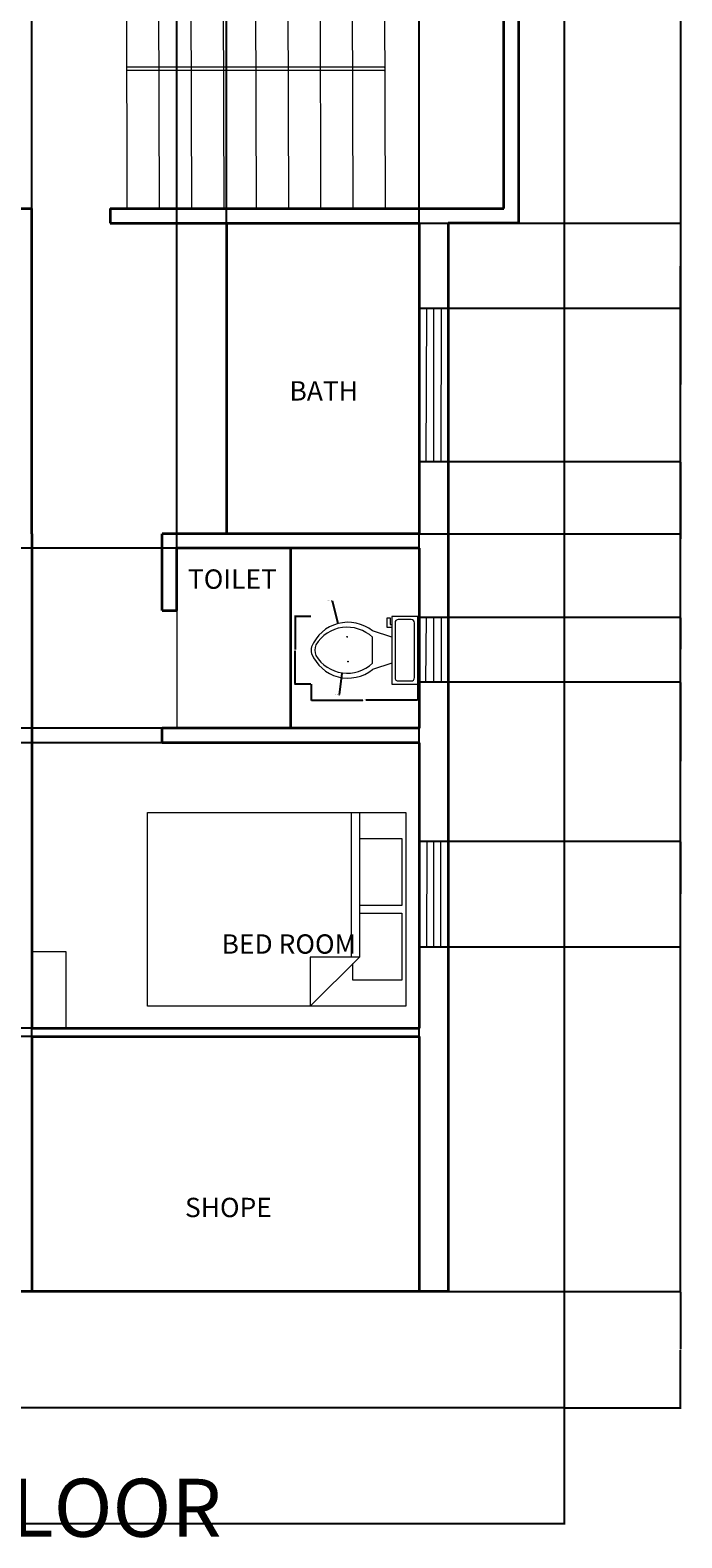
# Model space of a CAD drawing. Units: inches. Extents: x 2621 to 3621, y 1701 to 2465.
# Tile 2 of 6: x 2888 to 3090, y 1701 to 2169. Entities that reach past the tile are written whole.
import ezdxf

# ---------------------------------------------------------------- set-up
doc = ezdxf.new("R2010")
doc.units = ezdxf.units.IN
for name, color, linetype, lineweight in [('A-ANNO-DIMS', 2, 'Continuous', 18), ('A-ANNO-TEXT', 7, 'Continuous', 25), ('A-AREA-IDEN', 7, 'Continuous', 18), ('A-DOOR', 3, 'Continuous', 18), ('A-FLOR-CASE', 32, 'Continuous', 18), ('A-FLOR-FIXT', 9, 'Continuous', 18), ('A-FLOR-STRS', 30, 'Continuous', 18), ('A-FURN', 8, 'Continuous', 18), ('A-GLAZ', 4, 'Continuous', 18), ('A-WALL', 7, 'Continuous', 35), ('C-PROP', 8, 'Continuous', 25)]:
    doc.layers.add(name, color=color, linetype=linetype, lineweight=lineweight)
doc.styles.get("Standard").update_dxf_attribs({"font": 'arial.ttf'})
doc.dimstyles.get("Standard").update_dxf_attribs({"dimtxt": 0.18, "dimasz": 0.18, "dimexe": 0.18, "dimexo": 0.0625, "dimgap": 0.09, "dimtad": 0, "dimtih": 1, "dimtoh": 1, "dimdec": 4, "dimzin": 0, "dimdsep": 46, "dimtxsty": 'Standard', "dimcen": 0.09, "dimadec": 0, "dimazin": 0, "dimtfac": 1, "dimtdec": 4, "dimtofl": 0, "dimtmove": 0, "dimatfit": 3, "dimfxl": 1, "dimtolj": 1, "dimtzin": 0, "dimarcsym": 0})

# ---------------------------------------------------------------- blocks, each defined once
blk = doc.blocks.new('Bed - Queen')
for p, q in [((0, -80.00003), (0, 0)), ((0, 0), (59.99999, 0)), ((59.99999, 0), (59.99999, -80.00003)), ((7.99999, -1.2), (28.79998, -1.2)), ((7.99999, -14.4), (7.99999, -1.2)), ((28.79998, -1.2), (28.79998, -14.4)), ((31.19999, -1.2), (51.99999, -1.2)), ((31.19999, -14.4), (31.19999, -1.2)), ((51.99999, -1.2), (51.99999, -16.4)), ((0, -14.4), (44.8, -14.4)), ((44.8, -16.8), (0, -16.8)), ((59.99999, -29.6), (44.8, -14.4)), ((44.8, -14.4), (44.8, -29.6)), ((51.99999, -16.4), (46.79936, -16.4)), ((44.8, -29.6), (59.99999, -29.6)), ((59.99999, -80.00003), (0, -80.00003))]:
    blk.add_line(p, q)
blk = doc.blocks.new('Toilet - top')
for p, q in [((9.5, -6), (9.5, -2)), ((-10, -8.5), (-8, -8.5)), ((-10, -9.5), (-10, -8.5)), ((-8, -8.5), (-8, -8)), ((-7, -8), (-7, -9.5)), ((-4, -8), (-6, -14)), ((4, -8), (6, -14)), ((-7, -9.5), (-10, -9.5)), ((4, -14), (-4, -14))]:
    blk.add_line(p, q)
blk.add_lwpolyline([(10.5, -8), (10.5, 0), (-10.5, 0), (-10.5, -8)], close=True)
for points in [[(-9.5, -2), (-9.5, -6)], [(8.5, -1), (-8.5, -1)], [(-8.5, -7), (8.5, -7)]]:
    blk.add_lwpolyline(points)
for centre, radius, start, end in [((-8.62, -1.88), 0.884, 81.8699, 188.1301), ((8.62, -1.88), 0.884, 351.8699, 98.1301), ((-8.62, -6.12), 0.884, 171.8699, 278.1301), ((8.62, -6.12), 0.884, 261.8699, 8.1301), ((3.52, -21.58), 12.17, 141.4691, 247.9714), ((4.2, -21.82), 11.33, 136.3677, 238.9468), ((-3.52, -21.58), 12.17, 292.0284, 38.5307), ((-4.2, -21.82), 11.33, 301.053, 43.6321), ((0, -27.88), 4, 245.7318, 294.2682), ((0, -29), 4, 254.8605, 285.1395)]:
    blk.add_arc(centre, radius, start, end)
blk = doc.blocks.new('LOT-33X57')
for p, q in [((396, 684), (396, 0)), ((396, 0), (0, 0))]:
    blk.add_line(p, q)
blk = doc.blocks.new('STAIR-RETURN-FLIGHT')
for p, q in [((0.25, 0), (0, 86.58)), ((10.25, 0.03), (10, 86.61)), ((20.25, 0.06), (20, 86.64)), ((30.25, 0.09), (30, 86.67)), ((40.25, 0.12), (40, 86.7)), ((50.25, 0.15), (50, 86.73)), ((60.25, 0.18), (60, 86.76)), ((70.25, 0.2), (70, 86.79)), ((80.25, 0.23), (80, 86.82)), ((6.51, 44.03), (0.13, 44.03)), ((6.51, 43.03), (0.13, 43.03)), ((79.82, 44.03), (6.51, 44.03)), ((79.82, 43.03), (6.51, 43.03)), ((79.82, 44.03), (80.13, 44.03)), ((79.82, 43.03), (80.13, 43.03)), ((70.59, 0.23), (70.59, 0.06))]:
    blk.add_line(p, q)
blk = doc.blocks.new('*D33')
at = {"layer": 'A-ANNO-DIMS', "color": 0, "lineweight": -2, "transparency": 16777216}
for p, q in [((2975.04, 1965.73), (2975.04, 1960.65)), ((3008.09, 1965.73), (3008.09, 1960.65)), ((2975.22, 1960.83), (2991.1, 1960.83)), ((3007.91, 1960.83), (2992.03, 1960.83))]:
    blk.add_line(p, q, dxfattribs=at)
at = {"layer": 'A-ANNO-DIMS', "color": 0, "transparency": 16777216}
for points in [[(2975.22, 1960.86), (2975.22, 1960.8), (2975.04, 1960.83)], [(3007.91, 1960.86), (3007.91, 1960.8), (3008.09, 1960.83)]]:
    blk.add_solid(points, dxfattribs=at)
at = {"layer": 'Defpoints', "color": 0, "transparency": 16777216}
for p in [(2975.04, 1965.79), (3008.09, 1965.79), (3008.09, 1960.83)]:
    blk.add_point(p, dxfattribs=at)
at = {"layer": 'A-ANNO-DIMS', "color": 0, "transparency": 16777216, "insert": (2991.57, 1960.83), "char_height": 0.18, "attachment_point": 5}
blk.add_mtext('\\A1;WC 33', dxfattribs=at)
blk = doc.blocks.new('*D34')
at = {"layer": 'A-ANNO-DIMS', "color": 0, "lineweight": -2, "transparency": 16777216}
for p, q in [((2974.98, 1986.79), (2969.91, 1986.79)), ((2970.09, 1986.61), (2970.09, 1976.47)), ((2970.09, 1965.97), (2970.09, 1976.11)), ((2974.98, 1965.79), (2969.91, 1965.79))]:
    blk.add_line(p, q, dxfattribs=at)
at = {"layer": 'A-ANNO-DIMS', "color": 0, "transparency": 16777216}
for points in [[(2970.06, 1986.61), (2970.12, 1986.61), (2970.09, 1986.79)], [(2970.06, 1965.97), (2970.12, 1965.97), (2970.09, 1965.79)]]:
    blk.add_solid(points, dxfattribs=at)
at = {"layer": 'Defpoints', "color": 0, "transparency": 16777216}
for p in [(2975.04, 1986.79), (2970.09, 1965.79), (2975.04, 1965.79)]:
    blk.add_point(p, dxfattribs=at)
at = {"layer": 'A-ANNO-DIMS', "color": 0, "transparency": 16777216, "insert": (2970.09, 1976.29), "char_height": 0.18, "attachment_point": 5}
blk.add_mtext('\\A1;21', dxfattribs=at)
blk = doc.blocks.new('*D35')
at = {"layer": 'A-ANNO-DIMS', "color": 0, "lineweight": -2, "transparency": 16777216}
for p, q in [((2657.52, 1741.34), (2657.52, 1705.2)), ((3053.52, 1741.34), (3053.52, 1705.2)), ((2657.7, 1705.38), (2855.23, 1705.38)), ((3053.34, 1705.38), (2855.81, 1705.38))]:
    blk.add_line(p, q, dxfattribs=at)
at = {"layer": 'A-ANNO-DIMS', "color": 0, "transparency": 16777216}
for points in [[(2657.7, 1705.41), (2657.7, 1705.35), (2657.52, 1705.38)], [(3053.34, 1705.41), (3053.34, 1705.35), (3053.52, 1705.38)]]:
    blk.add_solid(points, dxfattribs=at)
at = {"layer": 'Defpoints', "color": 0, "transparency": 16777216}
for p in [(2657.52, 1741.4), (3053.52, 1741.4), (3053.52, 1705.38)]:
    blk.add_point(p, dxfattribs=at)
at = {"layer": 'A-ANNO-DIMS', "color": 0, "transparency": 16777216, "insert": (2855.52, 1705.38), "char_height": 0.18, "attachment_point": 5}
blk.add_mtext('\\A1;396', dxfattribs=at)
blk = doc.blocks.new('*D38')
at = {"layer": 'A-ANNO-DIMS', "color": 0, "lineweight": -2, "transparency": 16777216}
for p, q in [((3017.58, 2389.4), (3089.72, 2389.4)), ((3089.54, 2389.22), (3089.54, 2083.58)), ((3089.54, 1777.58), (3089.54, 2083.22)), ((3017.58, 1777.4), (3089.72, 1777.4))]:
    blk.add_line(p, q, dxfattribs=at)
at = {"layer": 'A-ANNO-DIMS', "color": 0, "transparency": 16777216}
for points in [[(3089.51, 2389.22), (3089.57, 2389.22), (3089.54, 2389.4)], [(3089.51, 1777.58), (3089.57, 1777.58), (3089.54, 1777.4)]]:
    blk.add_solid(points, dxfattribs=at)
at = {"layer": 'Defpoints', "color": 0, "transparency": 16777216}
for p in [(3017.52, 2389.4), (3089.54, 2389.4), (3017.52, 1777.4)]:
    blk.add_point(p, dxfattribs=at)
at = {"layer": 'A-ANNO-DIMS', "color": 0, "transparency": 16777216, "insert": (3089.54, 2083.4), "char_height": 0.18, "attachment_point": 5}
blk.add_mtext('\\A1;612', dxfattribs=at)
blk = doc.blocks.new('*D40')
at = {"layer": 'A-ANNO-DIMS', "color": 0, "lineweight": -2, "transparency": 16777216}
for p, q in [((3017.58, 1777.4), (3089.72, 1777.4)), ((3089.54, 1777.22), (3089.54, 1759.58)), ((3089.54, 1741.58), (3089.54, 1759.22)), ((3053.58, 1741.4), (3089.72, 1741.4))]:
    blk.add_line(p, q, dxfattribs=at)
at = {"layer": 'A-ANNO-DIMS', "color": 0, "transparency": 16777216}
for points in [[(3089.51, 1777.22), (3089.57, 1777.22), (3089.54, 1777.4)], [(3089.51, 1741.58), (3089.57, 1741.58), (3089.54, 1741.4)]]:
    blk.add_solid(points, dxfattribs=at)
at = {"layer": 'Defpoints', "color": 0, "transparency": 16777216}
for p in [(3017.52, 1777.4), (3089.54, 1777.4), (3053.52, 1741.4)]:
    blk.add_point(p, dxfattribs=at)
at = {"layer": 'A-ANNO-DIMS', "color": 0, "transparency": 16777216, "insert": (3089.54, 1759.4), "char_height": 0.18, "attachment_point": 5}
blk.add_mtext('\\A1;36', dxfattribs=at)
blk = doc.blocks.new('*D53')
at = {"layer": 'A-ANNO-DIMS', "color": 0, "lineweight": -2, "transparency": 16777216}
for p, q in [((2888.5, 1777.46), (2888.5, 2461.61)), ((2888.68, 2461.43), (2948.05, 2461.43)), ((3008.34, 2461.43), (2948.96, 2461.43)), ((3008.52, 1777.46), (3008.52, 2461.61))]:
    blk.add_line(p, q, dxfattribs=at)
at = {"layer": 'A-ANNO-DIMS', "color": 0, "transparency": 16777216}
for points in [[(2888.68, 2461.46), (2888.68, 2461.4), (2888.5, 2461.43)], [(3008.34, 2461.46), (3008.34, 2461.4), (3008.52, 2461.43)]]:
    blk.add_solid(points, dxfattribs=at)
at = {"layer": 'Defpoints', "color": 0, "transparency": 16777216}
for p in [(3008.52, 2461.43), (2888.5, 1777.4), (3008.52, 1777.4)]:
    blk.add_point(p, dxfattribs=at)
at = {"layer": 'A-ANNO-DIMS', "color": 0, "transparency": 16777216, "insert": (2948.51, 2461.43), "char_height": 0.18, "attachment_point": 5}
blk.add_mtext('\\A1;120.02', dxfattribs=at)
blk = doc.blocks.new('*D54')
at = {"layer": 'A-ANNO-DIMS', "color": 0, "lineweight": -2, "transparency": 16777216}
for p, q in [((3008.46, 1856.54), (2621.31, 1856.54)), ((2621.49, 1856.36), (2621.49, 1817.15)), ((2621.49, 1777.58), (2621.49, 1816.79)), ((3008.46, 1777.4), (2621.31, 1777.4))]:
    blk.add_line(p, q, dxfattribs=at)
at = {"layer": 'A-ANNO-DIMS', "color": 0, "transparency": 16777216}
for points in [[(2621.46, 1856.36), (2621.52, 1856.36), (2621.49, 1856.54)], [(2621.46, 1777.58), (2621.52, 1777.58), (2621.49, 1777.4)]]:
    blk.add_solid(points, dxfattribs=at)
at = {"layer": 'Defpoints', "color": 0, "transparency": 16777216}
for p in [(2621.49, 1856.54), (3008.52, 1856.54), (3008.52, 1777.4)]:
    blk.add_point(p, dxfattribs=at)
at = {"layer": 'A-ANNO-DIMS', "color": 0, "transparency": 16777216, "insert": (2621.49, 1816.97), "char_height": 0.18, "attachment_point": 5}
blk.add_mtext('\\A1;79.14', dxfattribs=at)
blk = doc.blocks.new('*D55')
at = {"layer": 'A-ANNO-DIMS', "color": 0, "lineweight": -2, "transparency": 16777216}
for p, q in [((3008.46, 1947.58), (2621.31, 1947.58)), ((2621.49, 1947.4), (2621.49, 1903.51)), ((2621.49, 1859.26), (2621.49, 1903.15)), ((3008.46, 1859.08), (2621.31, 1859.08))]:
    blk.add_line(p, q, dxfattribs=at)
at = {"layer": 'A-ANNO-DIMS', "color": 0, "transparency": 16777216}
for points in [[(2621.46, 1947.4), (2621.52, 1947.4), (2621.49, 1947.58)], [(2621.46, 1859.26), (2621.52, 1859.26), (2621.49, 1859.08)]]:
    blk.add_solid(points, dxfattribs=at)
at = {"layer": 'Defpoints', "color": 0, "transparency": 16777216}
for p in [(2621.49, 1947.58), (3008.52, 1947.58), (3008.52, 1859.08)]:
    blk.add_point(p, dxfattribs=at)
at = {"layer": 'A-ANNO-DIMS', "color": 0, "transparency": 16777216, "insert": (2621.49, 1903.33), "char_height": 0.18, "attachment_point": 5}
blk.add_mtext('\\A1;88.5', dxfattribs=at)
blk = doc.blocks.new('*D56')
at = {"layer": 'A-ANNO-DIMS', "color": 0, "lineweight": -2, "transparency": 16777216}
for p, q in [((2948.9, 2012.46), (2948.9, 2461.61)), ((2949.08, 2461.43), (2978.32, 2461.43)), ((3008.34, 2461.43), (2979.1, 2461.43)), ((3008.52, 2012.46), (3008.52, 2461.61))]:
    blk.add_line(p, q, dxfattribs=at)
at = {"layer": 'A-ANNO-DIMS', "color": 0, "transparency": 16777216}
for points in [[(2949.08, 2461.46), (2949.08, 2461.4), (2948.9, 2461.43)], [(3008.34, 2461.46), (3008.34, 2461.4), (3008.52, 2461.43)]]:
    blk.add_solid(points, dxfattribs=at)
at = {"layer": 'Defpoints', "color": 0, "transparency": 16777216}
for p in [(3008.52, 2461.43), (2948.9, 2012.4), (3008.52, 2012.4)]:
    blk.add_point(p, dxfattribs=at)
at = {"layer": 'A-ANNO-DIMS', "color": 0, "transparency": 16777216, "insert": (2978.71, 2461.43), "char_height": 0.18, "attachment_point": 5}
blk.add_mtext('\\A1;59.62', dxfattribs=at)
blk = doc.blocks.new('*D57')
at = {"layer": 'A-ANNO-DIMS', "color": 0, "lineweight": -2, "transparency": 16777216}
for p, q in [((2948.96, 2108.75), (3089.72, 2108.75)), ((3089.54, 2108.57), (3089.54, 2060.76)), ((3089.54, 2012.58), (3089.54, 2060.39)), ((2948.96, 2012.4), (3089.72, 2012.4))]:
    blk.add_line(p, q, dxfattribs=at)
at = {"layer": 'A-ANNO-DIMS', "color": 0, "transparency": 16777216}
for points in [[(3089.51, 2108.57), (3089.57, 2108.57), (3089.54, 2108.75)], [(3089.51, 2012.58), (3089.57, 2012.58), (3089.54, 2012.4)]]:
    blk.add_solid(points, dxfattribs=at)
at = {"layer": 'Defpoints', "color": 0, "transparency": 16777216}
for p in [(2948.9, 2108.75), (3089.54, 2108.75), (2948.9, 2012.4)]:
    blk.add_point(p, dxfattribs=at)
at = {"layer": 'A-ANNO-DIMS', "color": 0, "transparency": 16777216, "insert": (3089.54, 2060.58), "char_height": 0.18, "attachment_point": 5}
blk.add_mtext('\\A1;96.36', dxfattribs=at)
blk = doc.blocks.new('*D58')
at = {"layer": 'A-ANNO-DIMS', "color": 0, "lineweight": -2, "transparency": 16777216}
for p, q in [((2933.41, 2007.9), (2621.31, 2007.9)), ((2621.49, 2007.72), (2621.49, 1980.17)), ((2621.49, 1952.26), (2621.49, 1979.81)), ((2933.41, 1952.08), (2621.31, 1952.08))]:
    blk.add_line(p, q, dxfattribs=at)
at = {"layer": 'A-ANNO-DIMS', "color": 0, "transparency": 16777216}
for points in [[(2621.46, 2007.72), (2621.52, 2007.72), (2621.49, 2007.9)], [(2621.46, 1952.26), (2621.52, 1952.26), (2621.49, 1952.08)]]:
    blk.add_solid(points, dxfattribs=at)
at = {"layer": 'Defpoints', "color": 0, "transparency": 16777216}
for p in [(2621.49, 2007.9), (2933.47, 2007.9), (2933.47, 1952.08)]:
    blk.add_point(p, dxfattribs=at)
at = {"layer": 'A-ANNO-DIMS', "color": 0, "transparency": 16777216, "insert": (2621.49, 1979.99), "char_height": 0.18, "attachment_point": 5}
blk.add_mtext('\\A1;55.82', dxfattribs=at)
blk = doc.blocks.new('*D59')
at = {"layer": 'A-ANNO-DIMS', "color": 0, "lineweight": -2, "transparency": 16777216}
for p, q in [((2933.47, 2007.96), (2933.47, 2461.61)), ((2933.65, 2461.43), (2970.6, 2461.43)), ((3008.34, 2461.43), (2971.39, 2461.43)), ((3008.52, 2007.96), (3008.52, 2461.61))]:
    blk.add_line(p, q, dxfattribs=at)
at = {"layer": 'A-ANNO-DIMS', "color": 0, "transparency": 16777216}
for points in [[(2933.65, 2461.46), (2933.65, 2461.4), (2933.47, 2461.43)], [(3008.34, 2461.46), (3008.34, 2461.4), (3008.52, 2461.43)]]:
    blk.add_solid(points, dxfattribs=at)
at = {"layer": 'Defpoints', "color": 0, "transparency": 16777216}
for p in [(3008.52, 2461.43), (2933.47, 2007.9), (3008.52, 2007.9)]:
    blk.add_point(p, dxfattribs=at)
at = {"layer": 'A-ANNO-DIMS', "color": 0, "transparency": 16777216, "insert": (2971, 2461.43), "char_height": 0.18, "attachment_point": 5}
blk.add_mtext('\\A1;75.04', dxfattribs=at)
blk = doc.blocks.new('*D92')
at = {"layer": 'A-ANNO-DIMS', "color": 0, "lineweight": -2, "transparency": 16777216}
for p, q in [((3008.58, 1917.05), (3089.72, 1917.05)), ((3089.54, 1916.87), (3089.54, 1900.86)), ((3089.54, 1884.49), (3089.54, 1900.5)), ((3008.58, 1884.31), (3089.72, 1884.31))]:
    blk.add_line(p, q, dxfattribs=at)
at = {"layer": 'A-ANNO-DIMS', "color": 0, "transparency": 16777216}
for points in [[(3089.51, 1916.87), (3089.57, 1916.87), (3089.54, 1917.05)], [(3089.51, 1884.49), (3089.57, 1884.49), (3089.54, 1884.31)]]:
    blk.add_solid(points, dxfattribs=at)
at = {"layer": 'Defpoints', "color": 0, "transparency": 16777216}
for p in [(3008.52, 1917.05), (3089.54, 1917.05), (3008.52, 1884.31)]:
    blk.add_point(p, dxfattribs=at)
at = {"layer": 'A-ANNO-DIMS', "color": 0, "transparency": 16777216, "insert": (3089.54, 1900.68), "char_height": 0.18, "attachment_point": 5}
blk.add_mtext('\\A1;32.736', dxfattribs=at)
blk = doc.blocks.new('*D93')
at = {"layer": 'A-ANNO-DIMS', "color": 0, "lineweight": -2, "transparency": 16777216}
for p, q in [((3008.58, 1966.45), (3089.72, 1966.45)), ((3089.54, 1966.27), (3089.54, 1941.93)), ((3089.54, 1917.23), (3089.54, 1941.57)), ((3008.58, 1917.05), (3089.72, 1917.05))]:
    blk.add_line(p, q, dxfattribs=at)
at = {"layer": 'A-ANNO-DIMS', "color": 0, "transparency": 16777216}
for points in [[(3089.51, 1966.27), (3089.57, 1966.27), (3089.54, 1966.45)], [(3089.51, 1917.23), (3089.57, 1917.23), (3089.54, 1917.05)]]:
    blk.add_solid(points, dxfattribs=at)
at = {"layer": 'Defpoints', "color": 0, "transparency": 16777216}
for p in [(3008.52, 1966.45), (3089.54, 1966.45), (3008.52, 1917.05)]:
    blk.add_point(p, dxfattribs=at)
at = {"layer": 'A-ANNO-DIMS', "color": 0, "transparency": 16777216, "insert": (3089.54, 1941.75), "char_height": 0.18, "attachment_point": 5}
blk.add_mtext('\\A1;49.4', dxfattribs=at)
blk = doc.blocks.new('*D94')
at = {"layer": 'A-ANNO-DIMS', "color": 0, "lineweight": -2, "transparency": 16777216}
for p, q in [((3008.58, 1986.54), (3089.72, 1986.54)), ((3089.54, 1986.36), (3089.54, 1976.68)), ((3089.54, 1966.63), (3089.54, 1976.32)), ((3008.58, 1966.45), (3089.72, 1966.45))]:
    blk.add_line(p, q, dxfattribs=at)
at = {"layer": 'A-ANNO-DIMS', "color": 0, "transparency": 16777216}
for points in [[(3089.51, 1986.36), (3089.57, 1986.36), (3089.54, 1986.54)], [(3089.51, 1966.63), (3089.57, 1966.63), (3089.54, 1966.45)]]:
    blk.add_solid(points, dxfattribs=at)
at = {"layer": 'Defpoints', "color": 0, "transparency": 16777216}
for p in [(3008.52, 1986.54), (3089.54, 1986.54), (3008.52, 1966.45)]:
    blk.add_point(p, dxfattribs=at)
at = {"layer": 'A-ANNO-DIMS', "color": 0, "transparency": 16777216, "insert": (3089.54, 1976.5), "char_height": 0.18, "attachment_point": 5}
blk.add_mtext('\\A1;20.09', dxfattribs=at)
blk = doc.blocks.new('*D95')
at = {"layer": 'A-ANNO-DIMS', "color": 0, "lineweight": -2, "transparency": 16777216}
for p, q in [((3008.58, 2034.76), (3089.72, 2034.76)), ((3089.54, 2034.58), (3089.54, 2010.83)), ((3089.54, 1986.72), (3089.54, 2010.47)), ((3008.58, 1986.54), (3089.72, 1986.54))]:
    blk.add_line(p, q, dxfattribs=at)
at = {"layer": 'A-ANNO-DIMS', "color": 0, "transparency": 16777216}
for points in [[(3089.51, 2034.58), (3089.57, 2034.58), (3089.54, 2034.76)], [(3089.51, 1986.72), (3089.57, 1986.72), (3089.54, 1986.54)]]:
    blk.add_solid(points, dxfattribs=at)
at = {"layer": 'Defpoints', "color": 0, "transparency": 16777216}
for p in [(3008.52, 2034.76), (3089.54, 2034.76), (3008.52, 1986.54)]:
    blk.add_point(p, dxfattribs=at)
at = {"layer": 'A-ANNO-DIMS', "color": 0, "transparency": 16777216, "insert": (3089.54, 2010.65), "char_height": 0.18, "attachment_point": 5}
blk.add_mtext('\\A1;48.22', dxfattribs=at)
blk = doc.blocks.new('*D96')
at = {"layer": 'A-ANNO-DIMS', "color": 0, "lineweight": -2, "transparency": 16777216}
for p, q in [((3008.58, 2082.41), (3089.72, 2082.41)), ((3089.54, 2082.23), (3089.54, 2058.77)), ((3089.54, 2034.94), (3089.54, 2058.41)), ((3008.58, 2034.76), (3089.72, 2034.76))]:
    blk.add_line(p, q, dxfattribs=at)
at = {"layer": 'A-ANNO-DIMS', "color": 0, "transparency": 16777216}
for points in [[(3089.51, 2082.23), (3089.57, 2082.23), (3089.54, 2082.41)], [(3089.51, 2034.94), (3089.57, 2034.94), (3089.54, 2034.76)]]:
    blk.add_solid(points, dxfattribs=at)
at = {"layer": 'Defpoints', "color": 0, "transparency": 16777216}
for p in [(3008.52, 2082.41), (3089.54, 2082.41), (3008.52, 2034.76)]:
    blk.add_point(p, dxfattribs=at)
at = {"layer": 'A-ANNO-DIMS', "color": 0, "transparency": 16777216, "insert": (3089.54, 2058.59), "char_height": 0.18, "attachment_point": 5}
blk.add_mtext('\\A1;47.65', dxfattribs=at)
blk = doc.blocks.new('*D97')
at = {"layer": 'A-ANNO-DIMS', "color": 0, "lineweight": -2, "transparency": 16777216}
for p, q in [((3008.58, 2108.75), (3089.72, 2108.75)), ((3089.54, 2108.57), (3089.54, 2095.77)), ((3089.54, 2082.59), (3089.54, 2095.4)), ((3008.58, 2082.41), (3089.72, 2082.41))]:
    blk.add_line(p, q, dxfattribs=at)
at = {"layer": 'A-ANNO-DIMS', "color": 0, "transparency": 16777216}
for points in [[(3089.51, 2108.57), (3089.57, 2108.57), (3089.54, 2108.75)], [(3089.51, 2082.59), (3089.57, 2082.59), (3089.54, 2082.41)]]:
    blk.add_solid(points, dxfattribs=at)
at = {"layer": 'Defpoints', "color": 0, "transparency": 16777216}
for p in [(3008.52, 2108.75), (3089.54, 2108.75), (3008.52, 2082.41)]:
    blk.add_point(p, dxfattribs=at)
at = {"layer": 'A-ANNO-DIMS', "color": 0, "transparency": 16777216, "insert": (3089.54, 2095.58), "char_height": 0.18, "attachment_point": 5}
blk.add_mtext('\\A1;26.34', dxfattribs=at)
blk = doc.blocks.new('*D108')
at = {"layer": 'A-ANNO-DIMS', "color": 0, "lineweight": -2, "transparency": 16777216}
for p, q in [((2981.38, 1991.6), (2981.56, 1991.6)), ((2981.56, 1991.6), (2983.37, 1984.71)), ((2986.42, 1972.77), (2986.6, 1972.77)), ((2986.51, 1972.68), (2986.51, 1972.86))]:
    blk.add_line(p, q, dxfattribs=at)
at = {"layer": 'A-ANNO-DIMS', "color": 0, "transparency": 16777216}
blk.add_solid([(2983.4, 1984.72), (2983.34, 1984.71), (2983.42, 1984.54)], dxfattribs=at)
at = {"layer": 'Defpoints', "color": 0, "transparency": 16777216}
for p in [(2983.42, 1984.54), (2986.51, 1972.77)]:
    blk.add_point(p, dxfattribs=at)
at = {"layer": 'A-ANNO-DIMS', "color": 0, "transparency": 16777216, "insert": (2980.71, 1991.6), "char_height": 0.18, "attachment_point": 5}
blk.add_mtext('\\A1;2X R12.17', dxfattribs=at)
blk = doc.blocks.new('*D109')
at = {"layer": 'A-ANNO-DIMS', "color": 0, "lineweight": -2, "transparency": 16777216}
for p, q in [((2986.18, 1980.49), (2986.36, 1980.49)), ((2986.27, 1980.4), (2986.27, 1980.58)), ((2983.86, 1962.52), (2984.74, 1969.08)), ((2983.68, 1962.52), (2983.86, 1962.52))]:
    blk.add_line(p, q, dxfattribs=at)
at = {"layer": 'A-ANNO-DIMS', "color": 0, "transparency": 16777216}
blk.add_solid([(2984.71, 1969.09), (2984.77, 1969.08), (2984.76, 1969.26)], dxfattribs=at)
at = {"layer": 'Defpoints', "color": 0, "transparency": 16777216}
for p in [(2986.27, 1980.49), (2984.76, 1969.26)]:
    blk.add_point(p, dxfattribs=at)
at = {"layer": 'A-ANNO-DIMS', "color": 0, "transparency": 16777216, "insert": (2983, 1962.52), "char_height": 0.18, "attachment_point": 5}
blk.add_mtext('\\A1;2X R11.33', dxfattribs=at)

msp = doc.modelspace()

# ---------------------------------------------------------------- linework, layer by layer
at = {"layer": 'A-DOOR'}
msp.add_line((2933.4738, 1988.5937), (2933.4738, 1952.0771), dxfattribs=at)
at = {"layer": 'A-FLOR-CASE'}
msp.add_lwpolyline([(2888.495, 1859.0825), (2899.216, 1859.0825), (2899.216, 1882.7108), (2888.495, 1882.7108)], close=True, dxfattribs=at)
at = {"layer": 'A-GLAZ'}
for p, q in [((3010.7038, 2034.7604), (3010.9424, 2082.415)), ((3013.0184, 2082.415), (3013.0184, 2034.7604)), ((3015.3163, 2082.415), (3015.2368, 2034.7604)), ((3010.7349, 1986.5419), (3010.5077, 1966.4534)), ((3013.0184, 1986.5419), (3013.0184, 1966.4534)), ((3015.3938, 1986.5419), (3015.3938, 1966.4534)), ((3010.8891, 1917.049), (3010.7762, 1884.3132)), ((3013.0184, 1917.049), (3013.0184, 1884.3132)), ((3015.1972, 1917.049), (3015.1974, 1884.3132)), ((3008.5184, 1884.3132), (3017.5184, 1884.3132))]:
    msp.add_line(p, q, dxfattribs=at)
for points in [[(3008.5184, 2082.415), (3017.5184, 2082.415), (3017.5184, 2034.7604), (3008.5184, 2034.7604)], [(3008.5184, 1986.5419), (3017.5184, 1986.5419), (3017.5184, 1966.4534), (3008.5184, 1966.4534)], [(3008.5184, 1884.3132), (3017.5184, 1884.3132), (3017.5184, 1917.049), (3008.5184, 1917.049)]]:
    msp.add_lwpolyline(points, close=True, dxfattribs=at)
at = {"layer": 'A-WALL'}
for p, q in [((3039.3697, 2204.5707), (3039.3697, 2108.7527)), ((3034.7824, 2113.2527), (3034.7824, 2199.8382)), ((2883.995, 2113.2527), (2888.495, 2113.2527)), ((2888.495, 2012.3975), (2888.495, 2113.2527)), ((2912.8311, 2113.2527), (2912.8311, 2108.7527)), ((2912.8311, 2113.2527), (3017.5184, 2113.2527)), ((2912.8311, 2108.7527), (3008.5184, 2108.7527)), ((2948.9015, 2108.7527), (2948.9015, 2012.3975)), ((3008.5184, 2108.7527), (3008.5184, 2012.3975)), ((3017.5184, 2113.2527), (3034.7824, 2113.2527)), ((3039.3697, 2108.7527), (3017.5184, 2108.7527)), ((3017.5184, 2108.7527), (3017.5184, 1777.4015)), ((2888.495, 2012.3975), (2888.495, 2007.8975)), ((3008.5184, 2012.3975), (2928.9738, 2012.3975)), ((2928.9738, 2007.8975), (2928.9738, 2012.3975)), ((2888.495, 2007.8975), (2888.495, 1892.3987)), ((2928.9738, 1988.5937), (2928.9738, 2007.8975)), ((3008.5184, 2007.8975), (2933.4738, 2007.8975)), ((2933.4738, 1988.5937), (2933.4738, 2007.8975)), ((2968.7461, 1952.0771), (2968.7461, 2007.8975)), ((3008.5184, 2007.8975), (3008.5184, 1952.0771)), ((2928.9738, 1988.5937), (2933.4738, 1988.5937)), ((2928.9738, 1947.5771), (2928.9738, 1952.0771)), ((2933.4738, 1952.0771), (2928.9738, 1952.0771)), ((3008.5184, 1952.0771), (2933.4738, 1952.0771)), ((3008.5184, 1947.5771), (2928.9738, 1947.5771)), ((3008.5184, 1947.5771), (3008.5184, 1859.0825)), ((2888.495, 1892.3987), (2888.495, 1859.0825)), ((2888.495, 1859.0825), (3008.5184, 1859.0825)), ((2888.495, 1856.5401), (3008.5184, 1856.5401)), ((2888.495, 1856.5401), (2888.495, 1786.4015)), ((3008.5184, 1856.5401), (3008.5184, 1786.4015)), ((2888.495, 1786.4015), (2888.495, 1777.4015)), ((3008.5184, 1786.4015), (3008.5184, 1777.4015)), ((3017.5184, 1777.4015), (2883.995, 1777.4015))]:
    msp.add_line(p, q, dxfattribs=at)

# ---------------------------------------------------------------- block references
at = {"layer": 'A-FLOR-FIXT', "rotation": 270}
msp.add_blockref('Toilet - top', (3008.0882, 1976.2893), dxfattribs=at)
at = {"layer": 'A-FLOR-STRS'}
msp.add_blockref('STAIR-RETURN-FLIGHT', (2917.871, 2113.019), dxfattribs=at)
at = {"layer": 'A-FURN', "rotation": 270}
msp.add_blockref('Bed - Queen', (3004.4133, 1925.9517), dxfattribs=at)
at = {"layer": 'C-PROP'}
msp.add_blockref('LOT-33X57', (2657.518, 1741.402), dxfattribs=at)

# ---------------------------------------------------------------- texts
at = {"layer": 'A-ANNO-TEXT', "insert": (2759.8469, 1719.3538), "char_height": 18, "attachment_point": 1}
msp.add_mtext_dynamic_manual_height_columns('GROUND FLOOR', width=483.442651, gutter_width=12.5, heights=[0], dxfattribs=at)
at = {"layer": 'A-AREA-IDEN', "char_height": 6, "attachment_point": 1}
for s, width, insert in [('BATH', 12.444136, (2968.3648, 2059.7156)), ('TOILET', 9.68953, (2936.908, 2001.3427)), ('BED ROOM', 49.051461, (2947.3327, 1888.1756)), ('SHOPE', 21.347518, (2935.9947, 1806.4817))]:
    msp.add_mtext_dynamic_manual_height_columns(s, width=width, gutter_width=12.5, heights=[0], dxfattribs=dict(at, insert=insert))

# ---------------------------------------------------------------- dimensions: what is measured, and where the dimension line sits
at = {"layer": 'A-ANNO-DIMS'}
for base, p1, p2, override, picture, middle in [((3008.5184, 2461.427), (2888.495, 1777.4015), (3008.5184, 1777.4015), {"dimdec": 2, "dimlfac": 1, "dimrnd": 0, "dimzin": 0, "dimdsep": 46, "dimlunit": 2}, '*D53', (2948.5067, 2461.427)), ((3008.5184, 2461.427), (2933.4738, 2007.8975), (3008.5184, 2007.8975), {"dimdec": 2, "dimlfac": 1, "dimrnd": 0, "dimzin": 0, "dimdsep": 46, "dimlunit": 2}, '*D59', (2970.9961, 2461.427)), ((3008.5184, 2461.427), (2948.9015, 2012.3975), (3008.5184, 2012.3975), {"dimdec": 2, "dimlfac": 1, "dimrnd": 0, "dimzin": 0, "dimdsep": 46, "dimlunit": 2}, '*D56', (2978.71, 2461.427)), ((3053.5184, 1705.376), (2657.5184, 1741.4015), (3053.5184, 1741.4015), {"dimdec": 0, "dimlfac": 1, "dimrnd": 0, "dimzin": 0, "dimdsep": 46, "dimlunit": 2}, '*D35', (2855.5184, 1705.376))]:
    dim = msp.add_linear_dim(base=base, p1=p1, p2=p2, dimstyle='Standard', override=override, dxfattribs=at)
    dim.commit()
    dim.dimension.update_dxf_attribs({"geometry": picture, "text_midpoint": middle})
for base, p1, p2, angle, override, picture, middle in [((3089.5439, 2389.4015), (3017.5184, 1777.4015), (3017.5184, 2389.4015), 90, {"dimdec": 0, "dimlfac": 1, "dimrnd": 0, "dimzin": 0, "dimdsep": 46, "dimlunit": 2}, '*D38', (3089.5439, 2083.4015)), ((3089.5439, 2108.7527), (2948.9015, 2012.3975), (2948.9015, 2108.7527), 90, {"dimdec": 2, "dimlfac": 1, "dimrnd": 0, "dimzin": 0, "dimdsep": 46, "dimlunit": 2}, '*D57', (3089.5439, 2060.5751)), ((3089.5439, 2108.7527), (3008.5184, 2082.415), (3008.5184, 2108.7527), 90, {"dimdec": 2, "dimlfac": 1, "dimrnd": 0, "dimzin": 0, "dimdsep": 46, "dimlunit": 2}, '*D97', (3089.5439, 2095.5839)), ((3089.5439, 2082.415), (3008.5184, 2034.7604), (3008.5184, 2082.415), 90, {"dimdec": 2, "dimlfac": 1, "dimrnd": 0, "dimzin": 0, "dimdsep": 46, "dimlunit": 2}, '*D96', (3089.5439, 2058.5877)), ((3089.5439, 2034.7604), (3008.5184, 1986.5419), (3008.5184, 2034.7604), 90, {"dimdec": 2, "dimlfac": 1, "dimrnd": 0, "dimzin": 0, "dimdsep": 46, "dimlunit": 2}, '*D95', (3089.5439, 2010.6512)), ((2621.4929, 2007.8975), (2933.4738, 1952.0771), (2933.4738, 2007.8975), 90, {"dimdec": 2, "dimlfac": 1, "dimrnd": 0, "dimzin": 0, "dimdsep": 46, "dimlunit": 2}, '*D58', (2621.4929, 1979.9873)), ((2970.0851, 1965.7893), (2975.042, 1986.7893), (2975.042, 1965.7893), 270, {"dimdec": 0, "dimlfac": 1, "dimrnd": 0, "dimzin": 0, "dimdsep": 46, "dimlunit": 2}, '*D34', (2970.0851, 1976.2893)), ((3089.5439, 1986.5419), (3008.5184, 1966.4534), (3008.5184, 1986.5419), 90, {"dimdec": 2, "dimlfac": 1, "dimrnd": 0, "dimzin": 0, "dimdsep": 46, "dimlunit": 2}, '*D94', (3089.5439, 1976.4977)), ((3089.5439, 1966.4534), (3008.5184, 1917.049), (3008.5184, 1966.4534), 90, {"dimdec": 1, "dimlfac": 1, "dimrnd": 0, "dimzin": 0, "dimdsep": 46, "dimlunit": 2}, '*D93', (3089.5439, 1941.7512)), ((2621.4929, 1947.5771), (3008.5184, 1859.0825), (3008.5184, 1947.5771), 90, {"dimdec": 1, "dimlfac": 1, "dimrnd": 0, "dimzin": 0, "dimdsep": 46, "dimlunit": 2}, '*D55', (2621.4929, 1903.3298)), ((3089.5439, 1917.049), (3008.5184, 1884.3132), (3008.5184, 1917.049), 90, {"dimdec": 3, "dimlfac": 1, "dimrnd": 0, "dimzin": 0, "dimdsep": 46, "dimlunit": 2}, '*D92', (3089.5439, 1900.6811)), ((2621.4929, 1856.5401), (3008.5184, 1777.4015), (3008.5184, 1856.5401), 90, {"dimdec": 2, "dimlfac": 1, "dimrnd": 0, "dimzin": 0, "dimdsep": 46, "dimlunit": 2}, '*D54', (2621.4929, 1816.9708)), ((3089.5439, 1777.4015), (3053.5184, 1741.4015), (3017.5184, 1777.4015), 90, {"dimdec": 0, "dimlfac": 1, "dimrnd": 0, "dimzin": 0, "dimdsep": 46, "dimlunit": 2}, '*D40', (3089.5439, 1759.4015))]:
    dim = msp.add_linear_dim(base=base, p1=p1, p2=p2, angle=angle, dimstyle='Standard', override=override, dxfattribs=at)
    dim.commit()
    dim.dimension.update_dxf_attribs({"geometry": picture, "text_midpoint": middle})
for center, mpoint, picture, middle in [((2986.5078, 1972.7697), (2983.4159, 1984.5394), '*D108', (2980.706, 1991.6012)), ((2986.2709, 1980.4892), (2984.761, 1969.2611), '*D109', (2983.0003, 1962.5242))]:
    dim = msp.add_radius_dim(center=center, mpoint=mpoint, text='2X <>', dimstyle='Standard', override={"dimdec": 2, "dimlfac": 1, "dimrnd": 0, "dimzin": 0, "dimdsep": 46, "dimlunit": 2}, dxfattribs=at)
    dim.commit()
    dim.dimension.update_dxf_attribs({"geometry": picture, "text_midpoint": middle, "dimtype": 164})
dim = msp.add_linear_dim(base=(3008.0882, 1960.8324), p1=(2975.042, 1965.7893), p2=(3008.0882, 1965.7893), text='WC <>', dimstyle='Standard', override={"dimdec": 0, "dimlfac": 1, "dimrnd": 0, "dimzin": 0, "dimdsep": 46, "dimlunit": 2}, dxfattribs=at)
dim.commit()
dim.dimension.update_dxf_attribs({"geometry": '*D33', "text_midpoint": (2991.5651, 1960.8324)})

doc.saveas('drawing.dxf')
